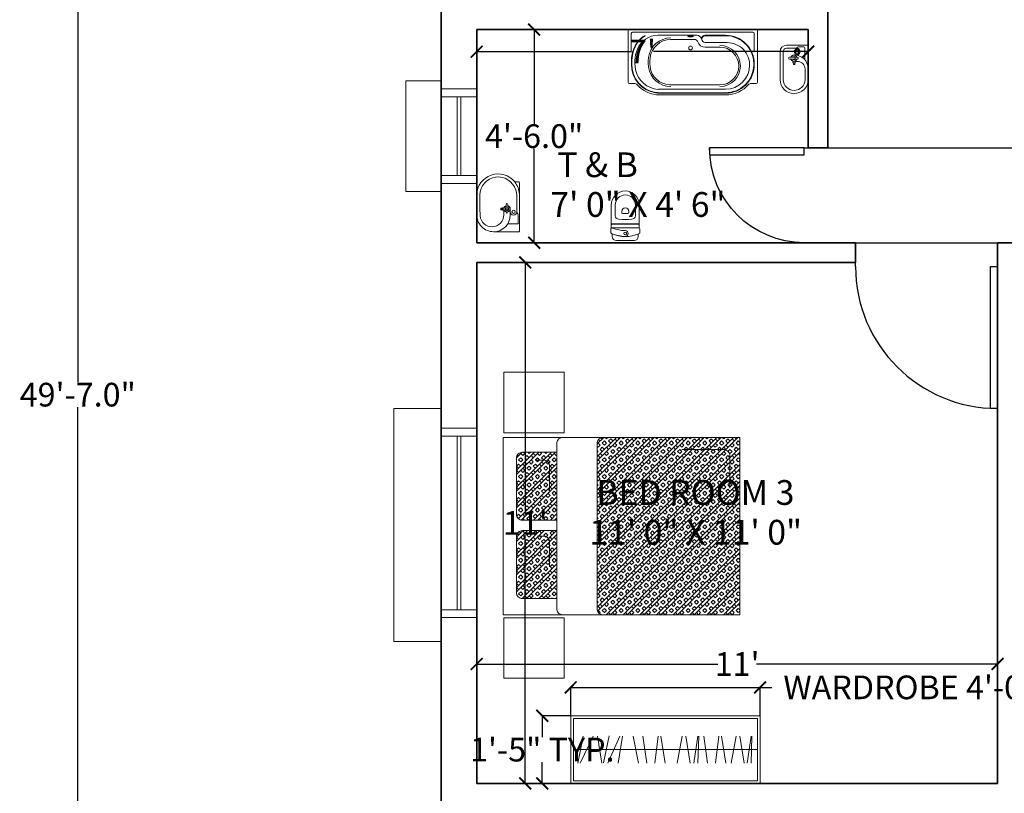
# Model space of a CAD drawing. Units: inches. Extents: x 844 to 2234, y 346 to 1084.
# Tile 2 of 93: x 844 to 1093, y 627 to 823. Entities that reach past the tile are written whole.
import ezdxf

# ---------------------------------------------------------------- set-up
doc = ezdxf.new("R2010")
doc.units = ezdxf.units.IN
doc.header["$MEASUREMENT"] = 0
for name, color, linetype, lineweight in [('A-ANNO-DIMS', 2, 'Continuous', 18), ('A-AREA-IDEN', 7, 'Continuous', 18), ('A-FLOR-FIXT', 8, 'Continuous', 18), ('A-WALL', 7, 'Continuous', 35), ('beds', 130, 'Continuous', 18), ('doors', 170, 'Continuous', 25), ('furniture', 8, 'Continuous', 18), ('windows', 1, 'Continuous', 18)]:
    doc.layers.add(name, color=color, linetype=linetype, lineweight=lineweight)
doc.styles.get("Standard").update_dxf_attribs({"font": 'arial.ttf'})
doc.dimstyles.get("Standard").update_dxf_attribs({"dimtxt": 6, "dimasz": 3, "dimexe": 0.18, "dimexo": 0.0625, "dimgap": 0.09, "dimtad": 0, "dimtih": 1, "dimtoh": 1, "dimdec": 1, "dimzin": 0, "dimdsep": 46, "dimlunit": 3, "dimtxsty": 'Standard', "dimblk": 'ARCHTICK', "dimcen": 0.09, "dimadec": 0, "dimazin": 0, "dimtfac": 1, "dimtdec": 1, "dimtofl": 0, "dimtmove": 0, "dimatfit": 3, "dimfxl": 1, "dimtolj": 1, "dimtzin": 0, "dimarcsym": 0})
pattern_1 = [(135, (-1377.70473, -125.71507), (-0.070710678, -0.070710678), []), (135, (-1377.68705, -125.69739), (-0.070710678, -0.070710678), []), (45, (-1377.70473, -125.71507), (-0.070710678, 0.070710678), [-0.025, 0.025]), (45, (-1377.72241, -125.69739), (-0.070710678, 0.070710678), [-0.025, 0.025]), (45, (-1377.74009, -125.67972), (-0.070710678, 0.070710678), [0.025, -0.025]), (45, (-1377.75776, -125.66204), (-0.070710678, 0.070710678), [0.025, -0.025]), (135, (-1377.66938, -125.67972), (-0.070710678, -0.070710678), [0.025, -0.025]), (135, (-1377.6517, -125.66204), (-0.070710678, -0.070710678), [0.025, -0.025])]

# ---------------------------------------------------------------- blocks, each defined once
blk = doc.blocks.new('*U2')
for p, q in [((0, 0), (0, -6)), ((36, 0), (36, -6))]:
    blk.add_line(p, q)
blk.add_lwpolyline([(0, 0), (0, 36), (1.75, 36), (1.75, 0)], close=True)
blk.add_arc((0, 0), 36, 0, 90)
blk = doc.blocks.new('*U4')
for p, q in [((0, 0), (0, -6)), ((24, 0), (24, -6))]:
    blk.add_line(p, q)
blk.add_lwpolyline([(0, 0), (0, 24), (1.75, 24), (1.75, 0)], close=True)
blk.add_arc((0, 0), 24, 0, 90)
blk = doc.blocks.new('MAT-P10')
h = blk.add_hatch()
h.set_pattern_fill('BOX', color=256, scale=0.1, angle=45, style=0)
h.set_pattern_definition(pattern_1)
h.paths.add_polyline_path([(-0.1565, 1.4605), (0.417, 1.4605), (0.417, 1.7513, 0.414214), (0.367, 1.8013), (-0.1065, 1.8013, 0.414214), (-0.1565, 1.7513)])
h.paths.add_polyline_path([(0.5052, 1.4604), (1.0792, 1.4604), (1.0792, 1.7513, 0.414214), (1.0292, 1.8013), (0.5552, 1.8013, 0.414214), (0.5052, 1.7513)])
h = blk.add_hatch()
h.set_pattern_fill('BOX', color=256, scale=0.1, angle=45, style=0)
h.set_pattern_definition(pattern_1)
edge = h.paths.add_edge_path()
edge.add_line((1.2049, -0.085), (1.2049, 1.0625))
edge.add_ellipse((1.1608, 1.0627), major_axis=(0, 0.0568), ratio=0.776379, start_angle=270, end_angle=360)
edge.add_line((1.1608, 1.1195), (-0.251, 1.1195))
edge.add_ellipse((-0.251, 1.0627), major_axis=(0, 0.0568), ratio=0.776379, start_angle=0, end_angle=88.13958)
edge.add_line((-0.2951, 1.0641), (-0.2951, -0.085))
edge.add_line((-0.2951, -0.085), (1.2049, -0.085))
for p, q in [((-0.251, 1.4605), (1.1608, 1.4604)), ((-0.251, 1.1195), (1.1608, 1.1195)), ((1.1017, 0.406), (1.1017, 0.0572)), ((1.0576, 0.0004), (0.7754, 0.0004))]:
    blk.add_line(p, q)
for points in [[(1.2049, -0.085), (-0.2951, -0.085), (-0.2951, 1.9151), (1.2049, 1.915)], [(-0.8301, 1.9091), (-0.3191, 1.9091), (-0.3191, 1.3981), (-0.8301, 1.3981)], [(1.2441, 1.9091), (1.755, 1.9091), (1.755, 1.3981), (1.2441, 1.3981)]]:
    blk.add_lwpolyline(points, close=True)
for points in [[(0.417, 1.4604), (0.417, 1.7513, 0.414214), (0.367, 1.8013), (-0.1065, 1.8013, 0.414214), (-0.1565, 1.7513), (-0.1565, 1.4604)], [(1.0792, 1.4603), (1.0792, 1.7513, 0.414214), (1.0292, 1.8013), (0.5552, 1.8013, 0.414214), (0.5052, 1.7513), (0.5052, 1.4604)], [(0.3702, 1.6242), (0.3702, 1.5715, -0.414214), (0.3202, 1.5215), (0.1113, 1.5215)], [(1.0117, 1.6438), (1.0117, 1.5715, -0.414214), (0.9617, 1.5215), (0.7528, 1.5215)]]:
    blk.add_lwpolyline(points, format="xyb")
at = {"extrusion": (0, 0, -1)}
for centre, start_param, end_param in [((-0.251, 1.4036), 4.712389, 6.283185), ((1.1608, 1.4036), 0, 1.570796), ((-0.251, 1.0627), 4.712389, 6.283185), ((1.1608, 1.0627), 0, 1.570796), ((1.0576, 0.0572), 1.570796, 3.141593), ((1.0576, 0.0572), 1.570796, 3.141593)]:
    blk.add_ellipse(centre, major_axis=(0, 0.0568), ratio=0.776379, start_param=start_param, end_param=end_param, dxfattribs=at)
blk = doc.blocks.new('A$C7A17768A')
for p, q in [((-2.8, 0), (0, 0)), ((-2.8, -1), (-2.8, 0)), ((0, -1), (0, 0)), ((-2.76, -0.04), (-0.04, -0.04)), ((-2.76, -0.96), (-2.76, -0.04)), ((-0.04, -0.96), (-0.04, -0.04)), ((-2.617, -0.3), (-2.694, -0.7)), ((-2.66, -0.7), (-2.466, -0.3)), ((-2.403, -0.3), (-2.342, -0.7)), ((-2.229, -0.296), (-2.317, -0.696)), ((-2.074, -0.3), (-2.25, -0.7)), ((-2.096, -0.7), (-2.033, -0.3)), ((-1.875, -0.3), (-1.796, -0.7)), ((-1.732, -0.3), (-1.675, -0.7)), ((-1.555, -0.7), (-1.507, -0.3)), ((-1.467, -0.3), (-1.403, -0.7)), ((-1.227, -0.7), (-1.151, -0.3)), ((-1.098, -0.3), (-1.034, -0.7)), ((-0.98, -0.7), (-0.921, -0.3)), ((-0.908, -0.3), (-0.919, -0.7)), ((-0.834, -0.3), (-0.777, -0.7)), ((-0.657, -0.7), (-0.61, -0.3)), ((-0.57, -0.3), (-0.505, -0.7)), ((-0.429, -0.7), (-0.353, -0.3)), ((-0.301, -0.3), (-0.237, -0.7)), ((-0.192, -0.7), (-0.133, -0.3)), ((-0.12, -0.3), (-0.131, -0.7)), ((-0.04, -0.5), (-2.716, -0.5)), ((-2.8, -1), (0, -1)), ((-2.76, -0.96), (-0.04, -0.96))]:
    blk.add_line(p, q)
blk = doc.blocks.new('2SABICO')
at = {"color": 0, "linetype": 'ByBlock'}
for p, q in [((0.478, 0.195), (0.089, 0.195)), ((0.478, 0.152), (0.089, 0.152)), ((0, 0.106), (0, 0)), ((0, 0), (0, -0.18)), ((0.043, -0.039), (0.043, 0.106)), ((0.135, 0), (0.135, -0.003)), ((0.168, 0.064), (0.168, -0.015)), ((0.192, 0.064), (0.192, -0.015)), ((0.221, 0.012), (0.222, 0.012)), ((0.223, 0.016), (0.223, -0.016)), ((0.224, 0.017), (0.245, 0.017)), ((0.246, 0.016), (0.246, -0.016)), ((0.25, 0.014), (0.246, 0.014)), ((0.26, 0.01), (0.268, 0.01)), ((0.268, -0.01), (0.268, 0.01)), ((0.268, 0.01), (0.269, 0.009)), ((0.269, -0.009), (0.269, 0.009)), ((0.023, -0.057), (0.023, -0.135)), ((0.135, 0), (0.135, -0.039)), ((0.168, -0.015), (0.192, -0.015)), ((0.168, -0.015), (0.168, -0.046)), ((0.192, -0.015), (0.192, -0.046)), ((0.221, -0.012), (0.222, -0.012)), ((0.224, -0.017), (0.245, -0.017)), ((0.225, -0.017), (0.225, -0.047)), ((0.25, -0.014), (0.246, -0.014)), ((0.26, -0.01), (0.268, -0.01)), ((0.268, -0.01), (0.269, -0.009)), ((0.015, -0.195), (0.478, -0.195)), ((0.038, -0.15), (0.179, -0.15)), ((0.33, -0.152), (0.478, -0.152))]:
    blk.add_line(p, q, dxfattribs=at)
for radius in [0.035, 0.023]:
    blk.add_circle((0.089, -0.039), radius, dxfattribs=at)
for centre, radius, start, end in [((0.089, 0.106), 0.089, 90, 180), ((0.089, 0.106), 0.046, 90, 180), ((0.478, 0), 0.195, 270, 90), ((0.478, 0), 0.152, 270, 90), ((0.18, 0), 0.045, 105.6643, 180), ((0.18, 0), 0.042, 106.8152, 252.6853), ((0.18, 0), 0.0235, 121.1327, 237.8651), ((0.18, 0.064), 0.0121, 0, 180), ((0.18, 0), 0.045, 17.0576, 74.3357), ((0.18, 0), 0.042, 287.3147, 73.1848), ((0.18, 0), 0.0235, 302.1349, 58.8673), ((0.221, 0.013), 0.001, 197.9471, 270), ((0.222, 0.013), 0.001, 270, 0), ((0.224, 0.016), 0.001, 90, 180), ((0.245, 0.016), 0.001, 0, 90), ((0.25, 0), 0.0143, 270, 90), ((0.041, -0.057), 0.018, 99.5941, 180), ((0.038, -0.135), 0.015, 180, 270), ((0.037, -0.033), 0.006, 279.5941, 0), ((0.089, -0.039), 0.046, 180, 360), ((0.326, -0.003), 0.191, 180, 270), ((0.18, -0.046), 0.0125, 180, 0), ((0.179, -0.14), 0.01, 270, 42.9682), ((0.221, -0.013), 0.001, 90, 162.0529), ((0.222, -0.013), 0.001, 0, 90), ((0.224, -0.016), 0.001, 180, 270), ((0.33, -0.047), 0.105, 180, 270), ((0.245, -0.016), 0.001, 270, 0), ((0.015, -0.18), 0.015, 180, 270)]:
    blk.add_arc(centre, radius, start, end, dxfattribs=at)
blk = doc.blocks.new('2SAINCO')
at = {"color": 0, "linetype": 'ByBlock'}
for p, q in [((0.06, 0.181), (0.085, 0.181)), ((0.114, 0.203), (0.165, 0.203)), ((0.496, 0.195), (0.178, 0.195)), ((0.18, -0.188), (0.18, 0.188)), ((0.231, 0.185), (0.231, -0.185)), ((0.234, 0.185), (0.234, -0.185)), ((0.496, 0.14), (0.347, 0.14)), ((0, -0.121), (0, 0.121)), ((0.394, 0.05), (0.407, 0.05)), ((0.394, -0.05), (0.407, -0.05)), ((0.06, -0.181), (0.085, -0.181)), ((0.114, -0.201), (0.165, -0.201)), ((0.114, -0.203), (0.165, -0.203)), ((0.496, -0.195), (0.178, -0.195)), ((0.496, -0.14), (0.347, -0.14))]:
    blk.add_line(p, q, dxfattribs=at)
blk.add_circle((0.1, 0), 0.02, dxfattribs=at)
for centre, radius, start, end in [((0.06, 0.121), 0.06, 90, 180), ((0.517, 0), 0.46, 155.909, 204.091), ((0.085, 0.196), 0.015, 270, 344.534), ((0.114, 0.188), 0.015, 90, 164.534), ((0.165, 0.188), 0.015, 0, 90), ((0.221, 0.185), 0.01, 0, 90), ((0.224, 0.185), 0.01, 0, 90), ((0.347, 0.09), 0.05, 90, 177.3546), ((0.496, 0), 0.195, 270, 90), ((0.496, 0), 0.14, 270, 90), ((0.1, 0), 0.0405, 360, 180), ((0.517, 0), 0.458, 180, 204.67), ((0.66, 0.008), 0.52, 180.891, 201.3823), ((2.295, 0), 2, 177.3546, 182.6454), ((0.677, 0), 0.3, 172.9459, 187.0541), ((0.394, 0.035), 0.015, 90, 172.9459), ((0.407, 0), 0.05, 270, 90), ((0.06, -0.121), 0.06, 180, 270), ((0.347, -0.09), 0.05, 182.6454, 270), ((0.394, -0.035), 0.015, 187.0541, 270), ((0.085, -0.196), 0.015, 15.466, 90), ((0.114, -0.188), 0.015, 195.466, 270), ((0.114, -0.188), 0.013, 195.466, 270), ((0.165, -0.188), 0.013, 270, 30), ((0.165, -0.188), 0.015, 270, 0), ((0.221, -0.185), 0.01, 270, 0), ((0.224, -0.185), 0.01, 270, 0)]:
    blk.add_arc(centre, radius, start, end, dxfattribs=at)
blk = doc.blocks.new('2SABACO')
at = {"color": 0}
for p, q in [((1.341, 0.831), (0.407, 0.831)), ((1.341, 0.91), (0.429, 0.91)), ((1.341, 0.885), (0.429, 0.885)), ((1.341, 0.879), (0.429, 0.879)), ((-0.015, 0.735), (-0.015, 0.015)), ((0, 0.75), (0.08, 0.75)), ((1.263, 0.769), (0.562, 0.769)), ((1.77, 0.75), (1.69, 0.75)), ((1.785, 0.015), (1.785, 0.735)), ((0.03, 0.302), (0.03, 0.053)), ((1.74, 0.053), (1.74, 0.286)), ((0.578, 0.139), (0.911, 0.139)), ((1.263, 0.245), (1.06, 0.245)), ((1.363, 0.181), (1.06, 0.181)), ((0, 0), (1.77, 0)), ((0.048, 0.035), (1.722, 0.035)), ((0.401, 0.08), (0.942, 0.08)), ((1.343, 0.086), (1.06, 0.086)), ((1.343, 0.079), (1.06, 0.079))]:
    blk.add_line(p, q, dxfattribs=at)
blk.add_circle((0.855, 0.256), 0.026, dxfattribs=at)
for centre, radius, start, end in [((0.428, 0.49), 0.395, 98.9726, 181.1954), ((0.428, 0.49), 0.389, 98.9726, 181.2301), ((0.425, 0.49), 0.342, 93.1008, 168.0202), ((0.429, 0.48), 0.43, 90, 139.2943), ((0.429, 0.48), 0.405, 90, 98.9726), ((0.429, 0.48), 0.399, 90, 98.9726), ((1.341, 0.48), 0.43, 40.7057, 90), ((1.341, 0.485), 0.401, 359.4627, 90), ((1.341, 0.485), 0.394, 3.5237, 90), ((1.341, 0.495), 0.336, 0, 90), ((0, 0.735), 0.015, 90, 180), ((0.08, 0.78), 0.03, 270, 319.2943), ((0.578, 0.481), 0.311, 90, 172.609), ((0.578, 0.481), 0.288, 93.3767, 172.609), ((1.263, 0.507), 0.285, 270, 90), ((1.263, 0.507), 0.262, 270, 90), ((1.69, 0.78), 0.03, 220.7057, 270), ((1.77, 0.735), 0.015, 0, 90), ((0.559, 0.454), 0.48, 163.1286, 202.3619), ((0.559, 0.454), 0.528, 177.0415, 202.3619), ((0.559, 0.454), 0.521, 177.0156, 202.3619), ((0.79, 0.454), 0.525, 172.609, 180), ((0.79, 0.454), 0.525, 180, 187.391), ((0.79, 0.454), 0.502, 172.609, 180), ((0.79, 0.454), 0.502, 180, 187.391), ((1.343, 0.477), 0.392, 270, 4.5675), ((1.343, 0.477), 0.398, 270, 0.539), ((1.363, 0.495), 0.314, 270, 2.2815), ((0.042, 0.302), 0.0116, 16.3184, 180.0001), ((0.578, 0.427), 0.311, 187.391, 270), ((0.578, 0.427), 0.288, 187.391, 270), ((1.718, 0.286), 0.0222, 0, 152.9966), ((0.401, 0.389), 0.357, 202.3619, 239.8287), ((0.401, 0.389), 0.351, 202.3619, 239.2093), ((0.401, 0.389), 0.309, 202.3619, 270), ((0.911, 0.183), 0.045, 270, 341.2369), ((1.06, 0.133), 0.112, 90, 161.2369), ((1.06, 0.133), 0.0475, 90, 270), ((0, 0.015), 0.015, 180, 270), ((0.048, 0.053), 0.018, 180, 270), ((0.559, 0.454), 0.48, 250.7818, 251.0555), ((0.821, 0.092), 0.00282, 119.7759, 180), ((0.821, 0.092), 0.00282, 180, 240.2241), ((0.837, 0.064), 0.0347, 103.3326, 119.7759), ((0.835, 0.025), 0.071, 96.5949, 102.1924), ((0.837, 0.12), 0.0347, 240.2241, 256.6674), ((0.847, -0.08), 0.177, 92.7417, 96.5949), ((0.848, 0.02), 0.0808, 95.6065, 103.3326), ((0.848, 0.164), 0.0808, 256.6674, 264.3935), ((0.855, -0.252), 0.349, 90, 92.7417), ((0.855, -0.053), 0.153, 90, 95.6065), ((0.855, 0.237), 0.153, 264.3935, 270), ((0.855, -0.053), 0.153, 84.3935, 90), ((0.855, -0.252), 0.349, 87.2583, 90), ((0.855, 0.237), 0.153, 270, 275.6065), ((0.862, 0.02), 0.0808, 76.6674, 84.3935), ((0.862, 0.164), 0.0808, 275.6065, 283.3326), ((0.863, -0.08), 0.177, 83.4051, 87.2583), ((0.873, 0.064), 0.0347, 60.2241, 76.6674), ((0.873, 0.12), 0.0347, 283.3326, 299.7759), ((0.875, 0.025), 0.071, 77.8076, 83.4051), ((0.889, 0.092), 0.00282, 360, 60.2241), ((0.889, 0.092), 0.00282, 299.7759, 360), ((0.942, 0.145), 0.065, 270, 349.4977), ((1.06, 0.133), 0.054, 180, 270), ((1.722, 0.053), 0.018, 270, 0), ((1.77, 0.015), 0.015, 270, 0)]:
    blk.add_arc(centre, radius, start, end, dxfattribs=at)
blk = doc.blocks.new('2SALACO2')
at = {"color": 0}
for p, q in [((0, 0), (-0.392, 0)), ((0.28, 0), (0, 0)), ((-0.402, -0.01), (-0.402, -0.36)), ((-0.293, -0.026), (-0.293, -0.15)), ((-0.283, -0.016), (-0.166, -0.016)), ((-0.169, -0.128), (-0.085, -0.128)), ((-0.112, -0.035), (-0.133, -0.035)), ((-0.124, -0.035), (0.09, -0.035)), ((0.29, -0.01), (0.29, -0.064)), ((-0.102, -0.219), (-0.169, -0.219)), ((-0.1, -0.161), (-0.131, -0.161)), ((-0.1, -0.186), (-0.131, -0.186)), ((-0.102, -0.217), (-0.102, -0.234)), ((-0.07, -0.216), (-0.101, -0.216)), ((-0.07, -0.235), (-0.101, -0.235)), ((-0.1, -0.161), (-0.1, -0.186)), ((-0.021, -0.161), (-0.1, -0.161)), ((-0.021, -0.186), (-0.1, -0.186)), ((-0.098, -0.214), (-0.098, -0.216)), ((-0.097, -0.239), (-0.098, -0.241)), ((-0.098, -0.241), (-0.098, -0.248)), ((-0.098, -0.241), (-0.073, -0.241)), ((-0.073, -0.248), (-0.098, -0.248)), ((-0.097, -0.235), (-0.097, -0.239)), ((-0.074, -0.239), (-0.097, -0.239)), ((-0.097, -0.248), (-0.097, -0.256)), ((-0.073, -0.256), (-0.097, -0.256)), ((-0.097, -0.256), (-0.094, -0.257)), ((-0.077, -0.257), (-0.094, -0.257)), ((-0.073, -0.256), (-0.077, -0.257)), ((-0.074, -0.235), (-0.074, -0.239)), ((-0.074, -0.239), (-0.073, -0.241)), ((-0.073, -0.214), (-0.073, -0.216)), ((-0.073, -0.241), (-0.073, -0.248)), ((-0.073, -0.248), (-0.073, -0.256)), ((-0.069, -0.217), (-0.069, -0.234))]:
    blk.add_line(p, q, dxfattribs=at)
blk.add_lwpolyline([(-0.402, -0.36, 0.423787), (-0.161, -0.593, 0.423787)], format="xyb", dxfattribs=at)
blk.add_circle((-0.124, -0.081), 0.023, dxfattribs=at)
for centre, radius, start, end in [((-0.392, -0.01), 0.01, 90, 180), ((0.28, -0.01), 0.01, 0, 90), ((-0.169, -0.36), 0.233, 90, 180), ((-0.283, -0.026), 0.01, 90, 180), ((-0.124, -0.081), 0.0462, 90, 270), ((-0.166, -0.046), 0.03, 31.2573, 90), ((-0.133, -0.026), 0.009, 211.2573, 270), ((-0.085, -0.173), 0.042, 16.8152, 162.6853), ((-0.085, -0.173), 0.0458, 15.3964, 90), ((0.09, -0.29), 0.255, 68.9449, 90), ((0.105, -0.295), 0.255, 271.0077, 72.4499), ((0.105, -0.297), 0.297, 271.4871, 51.4524), ((0.105, -0.297), 0.297, 51.4524, 87.1707), ((-0.169, -0.383), 0.164, 90, 265.4963), ((-0.285, -0.15), 0.008, 180, 299.1062), ((-0.131, -0.173), 0.0125, 90, 270), ((-0.085, -0.173), 0.042, 197.3147, 343.1848), ((-0.085, -0.173), 0.0235, 31.1327, 147.8651), ((-0.085, -0.173), 0.0235, 212.1349, 328.8673), ((-0.101, -0.217), 0.001, 90, 180), ((-0.101, -0.234), 0.001, 180, 270), ((-0.085, -0.173), 0.0458, 289.9182, 344.6036), ((-0.07, -0.217), 0.001, 0, 90), ((-0.07, -0.234), 0.001, 270, 0), ((-0.021, -0.173), 0.0121, 270, 90), ((0.021, 4.449), 5, 267.6742, 271.0081), ((-0.017, 4.405), 5, 268.3511, 271.4874)]:
    blk.add_arc(centre, radius, start, end, dxfattribs=at)
blk = doc.blocks.new('_ArchTick')
at = {"color": 0, "linetype": 'ByBlock', "const_width": 0.15}
blk.add_lwpolyline([(-0.5, -0.5), (0.5, 0.5)], dxfattribs=at)
blk = doc.blocks.new('*D31')
at = {"layer": 'A-ANNO-DIMS', "color": 0, "lineweight": -2, "transparency": 16777216}
for p, q in [((967.82, 761.31), (972.11, 761.31)), ((971.93, 761.31), (971.93, 698.41)), ((971.93, 629.31), (971.93, 692.21)), ((967.82, 629.31), (972.11, 629.31))]:
    blk.add_line(p, q, dxfattribs=at)
at = {"layer": 'Defpoints', "color": 0, "transparency": 16777216}
for p in [(967.76, 761.31), (967.76, 629.31), (971.93, 629.31)]:
    blk.add_point(p, dxfattribs=at)
at = {"layer": 'A-ANNO-DIMS', "color": 0, "lineweight": -2, "transparency": 16777216, "xscale": 3, "yscale": 3, "zscale": 3}
for p, rotation in [((971.93, 761.31), 90), ((971.93, 629.31), 270)]:
    blk.add_blockref('_ArchTick', p, dxfattribs=dict(at, rotation=rotation))
at = {"layer": 'A-ANNO-DIMS', "color": 0, "transparency": 16777216, "insert": (971.93, 695.31), "char_height": 6, "attachment_point": 5}
blk.add_mtext("\\A1;11'", dxfattribs=at)
blk = doc.blocks.new('*D32')
at = {"layer": 'A-ANNO-DIMS', "color": 0, "lineweight": -2, "transparency": 16777216}
for p, q in [((959.62, 659.63), (959.62, 659.75)), ((959.62, 659.57), (1020.72, 659.57)), ((1091.62, 659.57), (1030.51, 659.57)), ((1091.62, 659.63), (1091.62, 659.75))]:
    blk.add_line(p, q, dxfattribs=at)
at = {"layer": 'Defpoints', "color": 0, "transparency": 16777216}
for p in [(959.62, 659.57), (1091.62, 659.57), (1091.62, 659.57)]:
    blk.add_point(p, dxfattribs=at)
at = {"layer": 'A-ANNO-DIMS', "color": 0, "lineweight": -2, "transparency": 16777216, "xscale": 3, "yscale": 3, "zscale": 3, "rotation": 180}
blk.add_blockref('_ArchTick', (959.62, 659.57), dxfattribs=at)
at = {"layer": 'A-ANNO-DIMS', "color": 0, "lineweight": -2, "transparency": 16777216, "xscale": 3, "yscale": 3, "zscale": 3}
blk.add_blockref('_ArchTick', (1091.62, 659.57), dxfattribs=at)
at = {"layer": 'A-ANNO-DIMS', "color": 0, "transparency": 16777216, "insert": (1025.62, 659.57), "char_height": 6, "attachment_point": 5}
blk.add_mtext("\\A1;11'", dxfattribs=at)
blk = doc.blocks.new('*D37')
at = {"layer": 'A-ANNO-DIMS', "color": 0, "lineweight": -2, "transparency": 16777216}
for p, q in [((986.55, 820.31), (973.99, 820.31)), ((974.17, 820.31), (974.17, 796.46)), ((974.17, 766.31), (974.17, 790.16)), ((986.55, 766.31), (973.99, 766.31))]:
    blk.add_line(p, q, dxfattribs=at)
at = {"layer": 'Defpoints', "color": 0, "transparency": 16777216}
for p in [(986.62, 820.31), (974.17, 766.31), (986.62, 766.31)]:
    blk.add_point(p, dxfattribs=at)
at = {"layer": 'A-ANNO-DIMS', "color": 0, "lineweight": -2, "transparency": 16777216, "xscale": 3, "yscale": 3, "zscale": 3}
for p, rotation in [((974.17, 820.31), 90), ((974.17, 766.31), 270)]:
    blk.add_blockref('_ArchTick', p, dxfattribs=dict(at, rotation=rotation))
at = {"layer": 'A-ANNO-DIMS', "color": 0, "transparency": 16777216, "insert": (974.17, 793.31), "char_height": 6, "attachment_point": 5}
blk.add_mtext('\\A1;4\'-6.0"', dxfattribs=at)
blk = doc.blocks.new('*D38')
at = {"layer": 'A-ANNO-DIMS', "color": 0, "lineweight": -2, "transparency": 16777216}
for p, q in [((959.62, 818.26), (959.62, 814.55)), ((1043.62, 818.26), (1043.62, 814.55)), ((959.62, 814.73), (998.79, 814.73)), ((1043.62, 814.73), (1004.44, 814.73))]:
    blk.add_line(p, q, dxfattribs=at)
at = {"layer": 'Defpoints', "color": 0, "transparency": 16777216}
for p in [(959.62, 818.33), (1043.62, 818.33), (959.62, 814.73)]:
    blk.add_point(p, dxfattribs=at)
at = {"layer": 'A-ANNO-DIMS', "color": 0, "lineweight": -2, "transparency": 16777216, "xscale": 3, "yscale": 3, "zscale": 3, "rotation": 180}
blk.add_blockref('_ArchTick', (959.62, 814.73), dxfattribs=at)
at = {"layer": 'A-ANNO-DIMS', "color": 0, "lineweight": -2, "transparency": 16777216, "xscale": 3, "yscale": 3, "zscale": 3}
blk.add_blockref('_ArchTick', (1043.62, 814.73), dxfattribs=at)
at = {"layer": 'A-ANNO-DIMS', "color": 0, "transparency": 16777216, "insert": (1001.62, 814.73), "char_height": 6, "attachment_point": 5}
blk.add_mtext("\\A1;7'", dxfattribs=at)
blk = doc.blocks.new('*D56')
at = {"layer": 'A-ANNO-DIMS', "color": 0, "lineweight": -2, "transparency": 16777216}
for p, q in [((950.55, 1025.31), (858.33, 1025.31)), ((858.51, 1025.31), (858.51, 730.96)), ((858.51, 430.31), (858.51, 724.66)), ((950.55, 430.31), (858.33, 430.31))]:
    blk.add_line(p, q, dxfattribs=at)
at = {"layer": 'Defpoints', "color": 0, "transparency": 16777216}
for p in [(950.62, 1025.31), (858.51, 430.31), (950.62, 430.31)]:
    blk.add_point(p, dxfattribs=at)
at = {"layer": 'A-ANNO-DIMS', "color": 0, "lineweight": -2, "transparency": 16777216, "xscale": 3, "yscale": 3, "zscale": 3}
for p, rotation in [((858.51, 1025.31), 90), ((858.51, 430.31), 270)]:
    blk.add_blockref('_ArchTick', p, dxfattribs=dict(at, rotation=rotation))
at = {"layer": 'A-ANNO-DIMS', "color": 0, "transparency": 16777216, "insert": (858.51, 727.81), "char_height": 6, "attachment_point": 5}
blk.add_mtext('\\A1;49\'-7.0"', dxfattribs=at)
blk = doc.blocks.new('WIN-48IN')
for p, q in [((0, 9), (0, 21)), ((0, 21), (59, 21)), ((59, 9), (59, 21)), ((6, 9), (0, 9)), ((54, 9), (6, 9)), ((6, 9), (6, 0)), ((8, 9), (8, 0)), ((52, 0), (52, 9)), ((54, 0), (54, 9)), ((54, 9), (59, 9)), ((8, 5), (52, 5)), ((8, 4), (52, 4)), ((6, 0), (54, 0))]:
    blk.add_line(p, q)
blk = doc.blocks.new('WIN-24IN')
for p, q in [((9, 28), (0, 28)), ((0, 0), (0, 28)), ((9, 26), (9, 28)), ((18, 26), (9, 26)), ((9, 26), (9, 2)), ((18, 2), (18, 26)), ((18, 24), (9, 24)), ((13, 4), (13, 24)), ((14, 4), (14, 24)), ((9, 4), (18, 4)), ((9, 2), (18, 2)), ((9, 2), (9, 0)), ((9, 0), (0, 0))]:
    blk.add_line(p, q)
blk = doc.blocks.new('*D107')
at = {"layer": 'A-ANNO-DIMS', "color": 0, "lineweight": -2, "transparency": 16777216}
for p, q in [((983.44, 646.52), (983.44, 653.83)), ((1031.44, 646.52), (1031.44, 653.83)), ((983.44, 653.65), (1031.44, 653.65)), ((1031.44, 653.65), (1034.44, 653.65))]:
    blk.add_line(p, q, dxfattribs=at)
at = {"layer": 'Defpoints', "color": 0, "transparency": 16777216}
for p in [(1031.44, 653.65), (983.44, 646.45), (1031.44, 646.45)]:
    blk.add_point(p, dxfattribs=at)
at = {"layer": 'A-ANNO-DIMS', "color": 0, "lineweight": -2, "transparency": 16777216, "xscale": 3, "yscale": 3, "zscale": 3, "rotation": 180}
blk.add_blockref('_ArchTick', (983.44, 653.65), dxfattribs=at)
at = {"layer": 'A-ANNO-DIMS', "color": 0, "lineweight": -2, "transparency": 16777216, "xscale": 3, "yscale": 3, "zscale": 3}
blk.add_blockref('_ArchTick', (1031.44, 653.65), dxfattribs=at)
at = {"layer": 'A-ANNO-DIMS', "color": 0, "transparency": 16777216, "insert": (1078.79, 653.65), "char_height": 6, "attachment_point": 5}
blk.add_mtext('\\A1;WARDROBE 4\'-0" TYP.', dxfattribs=at)
blk = doc.blocks.new('*D108')
at = {"layer": 'A-ANNO-DIMS', "color": 0, "lineweight": -2, "transparency": 16777216}
for p, q in [((983.38, 646.45), (976.06, 646.45)), ((976.24, 646.45), (976.24, 641.04)), ((976.24, 629.31), (976.24, 634.73)), ((983.38, 629.31), (976.06, 629.31))]:
    blk.add_line(p, q, dxfattribs=at)
at = {"layer": 'Defpoints', "color": 0, "transparency": 16777216}
for p in [(976.24, 646.45), (983.44, 646.45), (983.44, 629.31)]:
    blk.add_point(p, dxfattribs=at)
at = {"layer": 'A-ANNO-DIMS', "color": 0, "lineweight": -2, "transparency": 16777216, "xscale": 3, "yscale": 3, "zscale": 3}
for p, rotation in [((976.24, 646.45), 90), ((976.24, 629.31), 270)]:
    blk.add_blockref('_ArchTick', p, dxfattribs=dict(at, rotation=rotation))
at = {"layer": 'A-ANNO-DIMS', "color": 0, "transparency": 16777216, "insert": (976.24, 637.88), "char_height": 6, "attachment_point": 5}
blk.add_mtext('\\A1;1\'-5" TYP.', dxfattribs=at)
blk = doc.blocks.new('*D149')
at = {"layer": 'A-ANNO-DIMS', "color": 0, "lineweight": -2, "transparency": 16777216}
for p, q in [((1043.68, 790.31), (1479.05, 790.31)), ((1478.87, 790.31), (1478.87, 781.46)), ((1478.87, 766.31), (1478.87, 775.16)), ((1043.68, 766.31), (1479.05, 766.31))]:
    blk.add_line(p, q, dxfattribs=at)
at = {"layer": 'Defpoints', "color": 0, "transparency": 16777216}
for p in [(1043.62, 790.31), (1478.87, 790.31), (1043.62, 766.31)]:
    blk.add_point(p, dxfattribs=at)
at = {"layer": 'A-ANNO-DIMS', "color": 0, "lineweight": -2, "transparency": 16777216, "xscale": 3, "yscale": 3, "zscale": 3}
for p, rotation in [((1478.87, 790.31), 90), ((1478.87, 766.31), 270)]:
    blk.add_blockref('_ArchTick', p, dxfattribs=dict(at, rotation=rotation))
at = {"layer": 'A-ANNO-DIMS', "color": 0, "transparency": 16777216, "insert": (1478.87, 778.31), "char_height": 6, "attachment_point": 5}
blk.add_mtext('\\A1;2\'-0"', dxfattribs=at)

msp = doc.modelspace()

# ---------------------------------------------------------------- linework, layer by layer
at = {"layer": 'A-WALL'}
for p, q in [((950.62, 1025.31), (950.62, 430.31)), ((1048.62, 879.31), (1048.62, 790.31)), ((959.62, 820.31), (1043.62, 820.31)), ((959.62, 820.31), (959.62, 766.31)), ((1043.62, 820.31), (1043.62, 790.31)), ((1048.62, 790.31), (1043.62, 790.31)), ((959.62, 766.31), (1043.62, 766.31)), ((1048.62, 766.31), (1043.62, 766.31)), ((1048.62, 766.31), (1055.62, 766.31)), ((1055.62, 761.31), (1055.62, 766.31)), ((1091.62, 761.31), (1091.62, 766.31)), ((1091.62, 766.31), (1096.62, 766.31)), ((959.62, 761.31), (1055.62, 761.31)), ((959.62, 761.31), (959.62, 629.31)), ((1091.62, 761.31), (1091.62, 629.31)), ((959.62, 629.31), (1091.62, 629.31))]:
    msp.add_line(p, q, dxfattribs=at)

# ---------------------------------------------------------------- block references
at = {"layer": 'A-FLOR-FIXT', "xscale": -18.21101258924898, "yscale": 18.21101258924898, "zscale": 18.21101258924898}
for name, p, rotation in [('2SABACO', (998.25, 820.31), 180), ('2SABICO', (1040.06, 816.34), 90), ('2SALACO2', (970.44, 776.41), 270), ('2SAINCO', (997.28, 766.83), 270)]:
    msp.add_blockref(name, p, dxfattribs=dict(at, rotation=rotation))
at = {"layer": 'beds', "xscale": 29.99962925113936, "yscale": 29.99962925113936, "zscale": 29.99962925113936, "rotation": 90}
msp.add_blockref('MAT-P10', (1023.75, 680.85), dxfattribs=at)
at = {"layer": 'doors', "xscale": -1, "rotation": 90}
msp.add_blockref('*U4', (1042.62, 790.31), dxfattribs=at)
at = {"layer": 'doors', "rotation": 180}
msp.add_blockref('*U2', (1091.62, 760.31), dxfattribs=at)
at = {"layer": 'furniture', "xscale": 17.14285714285603, "yscale": 17.14285714285603, "zscale": 17.14285714285603}
msp.add_blockref('A$C7A17768A', (1031.44, 646.45), dxfattribs=at)
at = {"layer": 'windows'}
msp.add_blockref('WIN-24IN', (941.62, 779.31), dxfattribs=at)
at = {"layer": 'windows', "rotation": 89.99999999999898}
msp.add_blockref('WIN-48IN', (959.62, 665.31), dxfattribs=at)

# ---------------------------------------------------------------- texts
at = {"layer": 'A-AREA-IDEN'}
for s, height, p in [('T & B', 6.269, (980.06, 782.93)), (' 7\' 0" X 4\' 6"', 6.2688, (976.36, 772.86)), ('BED ROOM 3', 6.269, (989.95, 699.89)), (' 11\' 0" X 11\' 0"', 6.2688, (986.25, 689.82))]:
    msp.add_text(s, height=height, dxfattribs=at).set_placement(p)

# ---------------------------------------------------------------- dimensions: what is measured, and where the dimension line sits
at = {"layer": 'A-ANNO-DIMS'}
for base, p1, p2, override, picture, middle in [((858.51, 430.31), (950.62, 1025.31), (950.62, 430.31), {"dimclrd": 0, "dimclre": 0, "dimclrt": 0}, '*D56', (858.51, 727.81)), ((974.17, 766.31), (986.62, 820.31), (986.62, 766.31), {"dimclrd": 0, "dimclre": 0, "dimclrt": 0}, '*D37', (974.17, 793.31)), ((1478.87, 790.31), (1043.62, 766.31), (1043.62, 790.31), {"dimdec": 1, "dimlfac": 1, "dimrnd": 0, "dimzin": 1, "dimdsep": 46, "dimlunit": 4, "dimfrac": 2}, '*D149', (1478.87, 778.31)), ((971.93, 629.31), (967.76, 761.31), (967.76, 629.31), {"dimclrd": 0, "dimclre": 0, "dimclrt": 0}, '*D31', (971.93, 695.31))]:
    dim = msp.add_linear_dim(base=base, p1=p1, p2=p2, angle=90, dimstyle='Standard', override=override, dxfattribs=at)
    dim.commit()
    dim.dimension.update_dxf_attribs({"geometry": picture, "text_midpoint": middle})
for base, p1, p2, picture, middle in [((959.62, 814.73), (1043.62, 818.33), (959.62, 818.33), '*D38', (1001.62, 814.73)), ((1091.62, 659.57), (959.62, 659.57), (1091.62, 659.57), '*D32', (1025.62, 659.57))]:
    dim = msp.add_linear_dim(base=base, p1=p1, p2=p2, dimstyle='Standard', override={"dimclrd": 0, "dimclre": 0, "dimclrt": 0}, dxfattribs=at)
    dim.commit()
    dim.dimension.update_dxf_attribs({"geometry": picture, "text_midpoint": middle})
dim = msp.add_linear_dim(base=(1031.44, 653.65), p1=(983.44, 646.45), p2=(1031.44, 646.45), text='WARDROBE <> TYP.', dimstyle='Standard', override={"dimdec": 1, "dimlfac": 1, "dimrnd": 0, "dimzin": 1, "dimdsep": 46, "dimlunit": 4, "dimfrac": 2}, dxfattribs=at)
dim.commit()
dim.dimension.update_dxf_attribs({"geometry": '*D107', "text_midpoint": (1078.79, 653.65)})
dim = msp.add_linear_dim(base=(976.24, 646.45), p1=(983.44, 629.31), p2=(983.44, 646.45), angle=90, text='<> TYP.', dimstyle='Standard', override={"dimdec": 1, "dimlfac": 1, "dimrnd": 0, "dimzin": 1, "dimdsep": 46, "dimlunit": 4, "dimfrac": 2}, dxfattribs=at)
dim.commit()
dim.dimension.update_dxf_attribs({"geometry": '*D108', "text_midpoint": (976.24, 637.88)})

doc.saveas('drawing.dxf')
